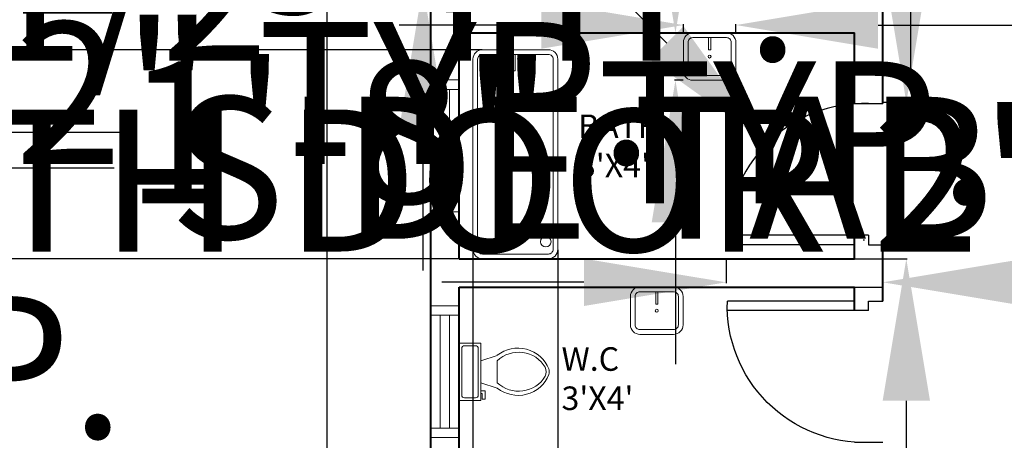
# Model space of a CAD drawing. Units: inches. Extents: x 7323 to 9737, y 2037 to 3322.
# Tile 8 of 19: x 8921 to 9130, y 2337 to 2426. Entities that reach past the tile are written whole.
import ezdxf

# ---------------------------------------------------------------- set-up
doc = ezdxf.new("R2010")
doc.units = ezdxf.units.IN
doc.header["$MEASUREMENT"] = 0
for name, color, linetype, lineweight in [('A-ANNO-DIMS', 2, 'Continuous', 18), ('A-AREA-IDEN', 7, 'Continuous', 18), ('A-DOOR', 4, 'Continuous', 25), ('A-FLOR-FIXT', 9, 'Continuous', 18), ('A-GLAZ', 4, 'Continuous', 18), ('A-WALL', 7, 'Continuous', 40)]:
    doc.layers.add(name, color=color, linetype=linetype, lineweight=lineweight)
doc.styles.get("Standard").update_dxf_attribs({"font": 'arial.ttf'})
doc.dimstyles.get("Standard").update_dxf_attribs({"dimtxt": 30.18, "dimasz": 30.18, "dimexe": 0.18, "dimexo": 0.0625, "dimgap": 0.09, "dimtad": 0, "dimtih": 1, "dimtoh": 1, "dimdec": 0, "dimzin": 0, "dimdsep": 46, "dimlunit": 3, "dimtxsty": 'Standard', "dimcen": 0.09, "dimadec": 0, "dimazin": 0, "dimtfac": 1, "dimtdec": 0, "dimtofl": 0, "dimtmove": 0, "dimatfit": 3, "dimfxl": 1, "dimtolj": 1, "dimtzin": 0, "dimarcsym": 0})

# ---------------------------------------------------------------- blocks, each defined once
blk = doc.blocks.new('*U2')
for p, q in [((9.5, -6), (9.5, -2)), ((-10, -8.5), (-8, -8.5)), ((-10, -9.5), (-10, -8.5)), ((-7, -9.5), (-10, -9.5)), ((-8, -8.5), (-8, -8)), ((-7, -8), (-7, -9.5)), ((-4, -8), (-6, -14)), ((4, -8), (6, -14)), ((4, -14), (-4, -14))]:
    blk.add_line(p, q)
blk.add_lwpolyline([(10.5, -8), (10.5, 0), (-10.5, 0), (-10.5, -8)], close=True)
for points in [[(-9.5, -2), (-9.5, -6)], [(8.5, -1), (-8.5, -1)], [(-8.5, -7), (8.5, -7)]]:
    blk.add_lwpolyline(points)
for centre, radius, start, end in [((-8.62, -1.88), 0.884, 81.8699, 188.1301), ((8.62, -1.88), 0.884, 351.8699, 98.1301), ((-8.62, -6.12), 0.884, 171.8699, 278.1301), ((8.62, -6.12), 0.884, 261.8699, 8.1301), ((3.52, -21.58), 12.17, 141.4691, 247.9714), ((4.2, -21.82), 11.33, 136.3677, 238.9468), ((-3.52, -21.58), 12.17, 292.0284, 38.5307), ((-4.2, -21.82), 11.33, 301.053, 43.6321), ((0, -27.88), 4, 245.7318, 294.2682), ((0, -29), 4, 254.8605, 285.1395)]:
    blk.add_arc(centre, radius, start, end)
blk = doc.blocks.new('*D11')
at = {"layer": 'A-ANNO-DIMS', "color": 0, "lineweight": -2, "transparency": 16777216}
for p, q in [((9007.88, 2687.3), (8985.8, 2687.3)), ((8985.98, 2657.12), (8985.98, 2458.79)), ((8985.98, 2229.48), (8985.98, 2427.8)), ((9007.88, 2199.3), (8985.8, 2199.3))]:
    blk.add_line(p, q, dxfattribs=at)
at = {"layer": 'A-ANNO-DIMS', "color": 0, "transparency": 16777216}
for points in [[(8980.95, 2657.12), (8991.01, 2657.12), (8985.98, 2687.3)], [(8980.95, 2229.48), (8991.01, 2229.48), (8985.98, 2199.3)]]:
    blk.add_solid(points, dxfattribs=at)
at = {"layer": 'Defpoints', "color": 0, "transparency": 16777216}
for p in [(9007.95, 2687.3), (8985.98, 2199.3), (9007.95, 2199.3)]:
    blk.add_point(p, dxfattribs=at)
at = {"layer": 'A-ANNO-DIMS', "color": 0, "transparency": 16777216, "insert": (8985.98, 2443.3), "char_height": 30.18, "attachment_point": 5}
blk.add_mtext('\\A1;40\'-8"', dxfattribs=at)
blk = doc.blocks.new('WIN-24')
for p, q in [((6, 28), (0, 28)), ((6, 26), (0, 26)), ((2, 26), (2, 2)), ((4, 26), (4, 2)), ((6, 2), (0, 2)), ((6, 0), (0, 0))]:
    blk.add_line(p, q)
blk = doc.blocks.new('DOOR-30')
for p, q in [((27.01, 33), (33.01, 33)), ((30.01, 5), (0.01, 5)), ((30.01, 5), (30.01, 3)), ((27.01, 3), (0.01, 3)), ((30.01, 3), (33.01, 3)), ((27.01, 0), (33.01, 0))]:
    blk.add_line(p, q)
blk.add_arc((29.01, 4), 29.02, 88.0251, 181.9749)
blk = doc.blocks.new('BASIN-WALL-MOUNT')
for points in [[(0, 8.06, -0.414214), (2, 10.06), (9.16, 10.06, -0.414214), (11.16, 8.06), (11.16, 2, -0.414214), (9.16, 0), (2, 0, -0.414214), (0, 2)], [(1, 8.06, -0.414214), (2, 9.06), (9.16, 9.06, -0.414214), (10.16, 8.06), (10.16, 2, -0.414214), (9.16, 1), (2, 1, -0.414214), (1, 2)]]:
    blk.add_lwpolyline(points, format="xyb", close=True)
blk.add_lwpolyline([(5.83, 9.06), (5.83, 9.06), (5.37, 9.06), (5.37, 9.06), (5.37, 6.45), (5.37, 6.45), (5.83, 6.45), (5.83, 6.45)], close=True)
blk.add_circle((5.58, 5.03), 0.311)
blk = doc.blocks.new('*D41')
at = {"layer": 'A-ANNO-DIMS', "color": 0, "lineweight": -2, "transparency": 16777216}
for p, q in [((8661.59, 2428.04), (8661.59, 2458.22)), ((8661.59, 2458.22), (8691.77, 2458.22)), ((8657.46, 2397.86), (8661.77, 2397.86)), ((8657.46, 2369.86), (8661.77, 2369.86)), ((8661.59, 2339.68), (8661.59, 2309.5))]:
    blk.add_line(p, q, dxfattribs=at)
at = {"layer": 'A-ANNO-DIMS', "color": 0, "transparency": 16777216}
for points in [[(8656.56, 2428.04), (8666.62, 2428.04), (8661.59, 2397.86)], [(8656.56, 2339.68), (8666.62, 2339.68), (8661.59, 2369.86)]]:
    blk.add_solid(points, dxfattribs=at)
at = {"layer": 'Defpoints', "color": 0, "transparency": 16777216}
for p in [(8657.39, 2397.86), (8661.59, 2397.86), (8657.39, 2369.86)]:
    blk.add_point(p, dxfattribs=at)
at = {"layer": 'A-ANNO-DIMS', "color": 0, "transparency": 16777216, "insert": (8945.06, 2458.22), "char_height": 30.18, "attachment_point": 5}
blk.add_mtext('\\A1;VENT WINDOW 2\'-4" TYP.', dxfattribs=at)
blk = doc.blocks.new('*D43')
at = {"layer": 'A-ANNO-DIMS', "color": 0, "lineweight": -2, "transparency": 16777216}
for p, q in [((9108.94, 2438.75), (9108.94, 2468.93)), ((9104.01, 2408.57), (9109.12, 2408.57)), ((9104.01, 2375.3), (9109.12, 2375.3)), ((9108.94, 2345.12), (9108.94, 2314.94))]:
    blk.add_line(p, q, dxfattribs=at)
at = {"layer": 'A-ANNO-DIMS', "color": 0, "transparency": 16777216}
for points in [[(9103.91, 2438.75), (9113.97, 2438.75), (9108.94, 2408.57)], [(9103.91, 2345.12), (9113.97, 2345.12), (9108.94, 2375.3)]]:
    blk.add_solid(points, dxfattribs=at)
at = {"layer": 'Defpoints', "color": 0, "transparency": 16777216}
for p in [(9103.95, 2408.57), (9108.94, 2408.57), (9103.95, 2375.3)]:
    blk.add_point(p, dxfattribs=at)
at = {"layer": 'A-ANNO-DIMS', "color": 0, "transparency": 16777216, "insert": (9108.94, 2391.93), "char_height": 30.18, "attachment_point": 5}
blk.add_mtext('\\A1;BATH DOOR 2\'-9 1/2" TYP.', dxfattribs=at)
blk = doc.blocks.new('*D44')
at = {"layer": 'A-ANNO-DIMS', "color": 0, "lineweight": -2, "transparency": 16777216}
for p, q in [((9070.67, 2375.23), (9070.67, 2370.12)), ((9103.95, 2375.23), (9103.95, 2370.12)), ((9040.49, 2370.3), (9010.31, 2370.3)), ((9134.13, 2370.3), (9164.31, 2370.3))]:
    blk.add_line(p, q, dxfattribs=at)
at = {"layer": 'A-ANNO-DIMS', "color": 0, "transparency": 16777216}
for points in [[(9040.49, 2375.33), (9040.49, 2365.27), (9070.67, 2370.3)], [(9134.13, 2375.33), (9134.13, 2365.27), (9103.95, 2370.3)]]:
    blk.add_solid(points, dxfattribs=at)
at = {"layer": 'Defpoints', "color": 0, "transparency": 16777216}
for p in [(9070.67, 2375.3), (9103.95, 2375.3), (9103.95, 2370.3)]:
    blk.add_point(p, dxfattribs=at)
at = {"layer": 'A-ANNO-DIMS', "color": 0, "transparency": 16777216, "insert": (9291.8, 2370.3), "char_height": 30.18, "attachment_point": 5}
blk.add_mtext('\\A1;2\'-9 1/2" TYP.', dxfattribs=at)
blk = doc.blocks.new('*D47')
at = {"layer": 'A-ANNO-DIMS', "color": 0, "lineweight": -2, "transparency": 16777216}
for p, q in [((8809.55, 2464.49), (8779.37, 2464.49)), ((8839.73, 2461.79), (8839.73, 2464.67)), ((8858.14, 2461.79), (8858.14, 2464.67)), ((8888.32, 2464.49), (8918.5, 2464.49))]:
    blk.add_line(p, q, dxfattribs=at)
at = {"layer": 'A-ANNO-DIMS', "color": 0, "transparency": 16777216}
for points in [[(8809.55, 2469.52), (8809.55, 2459.46), (8839.73, 2464.49)], [(8888.32, 2469.52), (8888.32, 2459.46), (8858.14, 2464.49)]]:
    blk.add_solid(points, dxfattribs=at)
at = {"layer": 'Defpoints', "color": 0, "transparency": 16777216}
for p in [(8858.14, 2464.49), (8839.73, 2461.73), (8858.14, 2461.73)]:
    blk.add_point(p, dxfattribs=at)
at = {"layer": 'A-ANNO-DIMS', "color": 0, "transparency": 16777216, "insert": (9164.9, 2464.49), "char_height": 30.18, "attachment_point": 5}
blk.add_mtext('\\A1;ARMCHAIR 1\'-6 1/2" TYP.', dxfattribs=at)
blk = doc.blocks.new('*D48')
at = {"layer": 'A-ANNO-DIMS', "color": 0, "lineweight": -2, "transparency": 16777216}
for p, q in [((8836.96, 2491.91), (8836.96, 2522.09)), ((8836.96, 2522.09), (8867.14, 2522.09)), ((8839.66, 2461.73), (8836.78, 2461.73)), ((8839.66, 2451.75), (8836.78, 2451.75)), ((8836.96, 2421.57), (8836.96, 2391.39))]:
    blk.add_line(p, q, dxfattribs=at)
at = {"layer": 'A-ANNO-DIMS', "color": 0, "transparency": 16777216}
for points in [[(8831.93, 2491.91), (8841.99, 2491.91), (8836.96, 2461.73)], [(8831.93, 2421.57), (8841.99, 2421.57), (8836.96, 2451.75)]]:
    blk.add_solid(points, dxfattribs=at)
at = {"layer": 'Defpoints', "color": 0, "transparency": 16777216}
for p in [(8836.96, 2461.73), (8839.73, 2461.73), (8839.73, 2451.75)]:
    blk.add_point(p, dxfattribs=at)
at = {"layer": 'A-ANNO-DIMS', "color": 0, "transparency": 16777216, "insert": (8970.94, 2522.09), "char_height": 30.18, "attachment_point": 5}
blk.add_mtext('\\A1;0\'-10" TYP.', dxfattribs=at)
blk = doc.blocks.new('*D53')
at = {"layer": 'A-ANNO-DIMS', "color": 0, "lineweight": -2, "transparency": 16777216}
for p, q in [((8857.03, 2503.93), (8857.03, 2511.24)), ((8905.03, 2503.93), (8905.03, 2511.24)), ((8826.85, 2511.06), (8796.67, 2511.06)), ((8935.21, 2511.06), (8965.39, 2511.06))]:
    blk.add_line(p, q, dxfattribs=at)
at = {"layer": 'A-ANNO-DIMS', "color": 0, "transparency": 16777216}
for points in [[(8826.85, 2516.09), (8826.85, 2506.03), (8857.03, 2511.06)], [(8935.21, 2516.09), (8935.21, 2506.03), (8905.03, 2511.06)]]:
    blk.add_solid(points, dxfattribs=at)
at = {"layer": 'Defpoints', "color": 0, "transparency": 16777216}
for p in [(8905.03, 2511.06), (8857.03, 2503.86), (8905.03, 2503.86)]:
    blk.add_point(p, dxfattribs=at)
at = {"layer": 'A-ANNO-DIMS', "color": 0, "transparency": 16777216, "insert": (9261.3, 2511.06), "char_height": 30.18, "attachment_point": 5}
blk.add_mtext('\\A1;INTERIOR WINDOW 4\'-0" TYP.', dxfattribs=at)
blk = doc.blocks.new('*D55')
at = {"layer": 'A-ANNO-DIMS', "color": 0, "lineweight": -2, "transparency": 16777216}
for p, q in [((9265.38, 2351.3), (9282, 2351.3)), ((9281.82, 2321.12), (9281.82, 2311.99)), ((9281.82, 2271.48), (9281.82, 2280.6)), ((9265.38, 2241.3), (9282, 2241.3))]:
    blk.add_line(p, q, dxfattribs=at)
at = {"layer": 'A-ANNO-DIMS', "color": 0, "transparency": 16777216}
for points in [[(9276.79, 2321.12), (9286.85, 2321.12), (9281.82, 2351.3)], [(9276.79, 2271.48), (9286.85, 2271.48), (9281.82, 2241.3)]]:
    blk.add_solid(points, dxfattribs=at)
at = {"layer": 'Defpoints', "color": 0, "transparency": 16777216}
for p in [(9265.32, 2351.3), (9281.82, 2351.3), (9265.32, 2241.3)]:
    blk.add_point(p, dxfattribs=at)
at = {"layer": 'A-ANNO-DIMS', "color": 0, "transparency": 16777216, "insert": (9281.82, 2296.3), "char_height": 30.18, "attachment_point": 5}
blk.add_mtext('\\A1;STAIR FLIGHT 9\'-2" TYP.', dxfattribs=at)
blk = doc.blocks.new('*D59')
at = {"layer": 'A-ANNO-DIMS', "color": 0, "lineweight": -2, "transparency": 16777216}
for p, q in [((9064.67, 2473.96), (9064.67, 2467.95)), ((9103.95, 2473.96), (9103.95, 2467.95)), ((9034.49, 2468.13), (9004.31, 2468.13)), ((9134.13, 2468.13), (9164.31, 2468.13))]:
    blk.add_line(p, q, dxfattribs=at)
at = {"layer": 'A-ANNO-DIMS', "color": 0, "transparency": 16777216}
for points in [[(9034.49, 2473.16), (9034.49, 2463.1), (9064.67, 2468.13)], [(9134.13, 2473.16), (9134.13, 2463.1), (9103.95, 2468.13)]]:
    blk.add_solid(points, dxfattribs=at)
at = {"layer": 'Defpoints', "color": 0, "transparency": 16777216}
for p in [(9064.67, 2474.02), (9103.95, 2474.02), (9103.95, 2468.13)]:
    blk.add_point(p, dxfattribs=at)
at = {"layer": 'A-ANNO-DIMS', "color": 0, "transparency": 16777216, "insert": (9458.35, 2468.13), "char_height": 30.18, "attachment_point": 5}
blk.add_mtext('\\A1;KITCHEN DOOR 3\'-3 1/2" TYP.', dxfattribs=at)
blk = doc.blocks.new('*D60')
at = {"layer": 'A-ANNO-DIMS', "color": 0, "lineweight": -2, "transparency": 16777216}
for p, q in [((9109.84, 2540.48), (9109.84, 2570.66)), ((9104.01, 2510.3), (9110.02, 2510.3)), ((9104.01, 2474.02), (9110.02, 2474.02)), ((9109.84, 2443.84), (9109.84, 2413.66))]:
    blk.add_line(p, q, dxfattribs=at)
at = {"layer": 'A-ANNO-DIMS', "color": 0, "transparency": 16777216}
for points in [[(9104.81, 2540.48), (9114.87, 2540.48), (9109.84, 2510.3)], [(9104.81, 2443.84), (9114.87, 2443.84), (9109.84, 2474.02)]]:
    blk.add_solid(points, dxfattribs=at)
at = {"layer": 'Defpoints', "color": 0, "transparency": 16777216}
for p in [(9103.95, 2510.3), (9109.84, 2510.3), (9103.95, 2474.02)]:
    blk.add_point(p, dxfattribs=at)
at = {"layer": 'A-ANNO-DIMS', "color": 0, "transparency": 16777216, "insert": (9109.84, 2492.16), "char_height": 30.18, "attachment_point": 5}
blk.add_mtext('\\A1;3\'-0 1/2" TYP.', dxfattribs=at)
blk = doc.blocks.new('*D63')
at = {"layer": 'A-ANNO-DIMS', "color": 0, "lineweight": -2, "transparency": 16777216}
for p, q in [((8744.72, 2466.22), (8744.72, 2496.4)), ((8744.72, 2496.4), (8774.9, 2496.4)), ((8741.46, 2436.04), (8744.9, 2436.04)), ((8741.46, 2413.86), (8744.9, 2413.86)), ((8744.72, 2383.68), (8744.72, 2353.5))]:
    blk.add_line(p, q, dxfattribs=at)
at = {"layer": 'A-ANNO-DIMS', "color": 0, "transparency": 16777216}
for points in [[(8739.69, 2466.22), (8749.75, 2466.22), (8744.72, 2436.04)], [(8739.69, 2383.68), (8749.75, 2383.68), (8744.72, 2413.86)]]:
    blk.add_solid(points, dxfattribs=at)
at = {"layer": 'Defpoints', "color": 0, "transparency": 16777216}
for p in [(8741.39, 2436.04), (8744.72, 2436.04), (8741.39, 2413.86)]:
    blk.add_point(p, dxfattribs=at)
at = {"layer": 'A-ANNO-DIMS', "color": 0, "transparency": 16777216, "insert": (9003.76, 2496.4), "char_height": 30.18, "attachment_point": 5}
blk.add_mtext('\\A1;APPLIANCE 1\'-10" TYP.', dxfattribs=at)
blk = doc.blocks.new('*D64')
at = {"layer": 'A-ANNO-DIMS', "color": 0, "lineweight": -2, "transparency": 16777216}
for p, q in [((8719.69, 2413.8), (8719.69, 2410.36)), ((8741.39, 2413.8), (8741.39, 2410.36)), ((8689.51, 2410.54), (8659.33, 2410.54)), ((8771.57, 2410.54), (8801.75, 2410.54))]:
    blk.add_line(p, q, dxfattribs=at)
at = {"layer": 'A-ANNO-DIMS', "color": 0, "transparency": 16777216}
for points in [[(8689.51, 2415.57), (8689.51, 2405.51), (8719.69, 2410.54)], [(8771.57, 2415.57), (8771.57, 2405.51), (8741.39, 2410.54)]]:
    blk.add_solid(points, dxfattribs=at)
at = {"layer": 'Defpoints', "color": 0, "transparency": 16777216}
for p in [(8719.69, 2413.86), (8741.39, 2413.86), (8741.39, 2410.54)]:
    blk.add_point(p, dxfattribs=at)
at = {"layer": 'A-ANNO-DIMS', "color": 0, "transparency": 16777216, "insert": (8927.57, 2410.54), "char_height": 30.18, "attachment_point": 5}
blk.add_mtext('\\A1;1\'-9 1/2" TYP.', dxfattribs=at)
blk = doc.blocks.new('*D67')
at = {"layer": 'A-ANNO-DIMS', "color": 0, "lineweight": -2, "transparency": 16777216}
for p, q in [((9145.07, 2308.82), (9145.07, 2339)), ((9150.37, 2278.64), (9144.89, 2278.64)), ((9150.37, 2242.89), (9144.89, 2242.89)), ((9145.07, 2212.71), (9145.07, 2182.53))]:
    blk.add_line(p, q, dxfattribs=at)
at = {"layer": 'A-ANNO-DIMS', "color": 0, "transparency": 16777216}
for points in [[(9140.04, 2308.82), (9150.1, 2308.82), (9145.07, 2278.64)], [(9140.04, 2212.71), (9150.1, 2212.71), (9145.07, 2242.89)]]:
    blk.add_solid(points, dxfattribs=at)
at = {"layer": 'Defpoints', "color": 0, "transparency": 16777216}
for p in [(9145.07, 2278.64), (9150.44, 2278.64), (9150.44, 2242.89)]:
    blk.add_point(p, dxfattribs=at)
at = {"layer": 'A-ANNO-DIMS', "color": 0, "transparency": 16777216, "insert": (9145.07, 2260.76), "char_height": 30.18, "attachment_point": 5}
blk.add_mtext('\\A1;TV UNIT 2\'-11 1/2" TYP.', dxfattribs=at)
blk = doc.blocks.new('*D68')
at = {"layer": 'A-ANNO-DIMS', "color": 0, "lineweight": -2, "transparency": 16777216}
for p, q in [((9120.26, 2284), (9090.08, 2284)), ((9150.44, 2278.7), (9150.44, 2284.18)), ((9163.95, 2278.7), (9163.95, 2284.18)), ((9194.13, 2284), (9224.31, 2284))]:
    blk.add_line(p, q, dxfattribs=at)
at = {"layer": 'A-ANNO-DIMS', "color": 0, "transparency": 16777216}
for points in [[(9120.26, 2289.03), (9120.26, 2278.97), (9150.44, 2284)], [(9194.13, 2289.03), (9194.13, 2278.97), (9163.95, 2284)]]:
    blk.add_solid(points, dxfattribs=at)
at = {"layer": 'Defpoints', "color": 0, "transparency": 16777216}
for p in [(9163.95, 2284), (9150.44, 2278.64), (9163.95, 2278.64)]:
    blk.add_point(p, dxfattribs=at)
at = {"layer": 'A-ANNO-DIMS', "color": 0, "transparency": 16777216, "insert": (9350.12, 2284), "char_height": 30.18, "attachment_point": 5}
blk.add_mtext('\\A1;1\'-1 1/2" TYP.', dxfattribs=at)
blk = doc.blocks.new('*D69')
at = {"layer": 'A-ANNO-DIMS', "color": 0, "lineweight": -2, "transparency": 16777216}
for p, q in [((8836.58, 2472.89), (8836.58, 2503.07)), ((8836.58, 2503.07), (8866.76, 2503.07)), ((8839.88, 2442.71), (8836.4, 2442.71)), ((8839.88, 2420.33), (8836.4, 2420.33)), ((8836.58, 2390.15), (8836.58, 2359.97))]:
    blk.add_line(p, q, dxfattribs=at)
at = {"layer": 'A-ANNO-DIMS', "color": 0, "transparency": 16777216}
for points in [[(8831.55, 2472.89), (8841.61, 2472.89), (8836.58, 2442.71)], [(8831.55, 2390.15), (8841.61, 2390.15), (8836.58, 2420.33)]]:
    blk.add_solid(points, dxfattribs=at)
at = {"layer": 'Defpoints', "color": 0, "transparency": 16777216}
for p in [(8836.58, 2442.71), (8839.94, 2442.71), (8839.94, 2420.33)]:
    blk.add_point(p, dxfattribs=at)
at = {"layer": 'A-ANNO-DIMS', "color": 0, "transparency": 16777216, "insert": (9169.54, 2503.07), "char_height": 30.18, "attachment_point": 5}
blk.add_mtext('\\A1;COFFEE TABLE 1\'-10 1/2" TYP.', dxfattribs=at)
blk = doc.blocks.new('*D70')
at = {"layer": 'A-ANNO-DIMS', "color": 0, "lineweight": -2, "transparency": 16777216}
for p, q in [((8809.76, 2446.06), (8779.58, 2446.06)), ((8839.94, 2442.77), (8839.94, 2446.24)), ((8855.74, 2442.77), (8855.74, 2446.24)), ((8885.92, 2446.06), (8916.1, 2446.06))]:
    blk.add_line(p, q, dxfattribs=at)
at = {"layer": 'A-ANNO-DIMS', "color": 0, "transparency": 16777216}
for points in [[(8809.76, 2451.09), (8809.76, 2441.03), (8839.94, 2446.06)], [(8885.92, 2451.09), (8885.92, 2441.03), (8855.74, 2446.06)]]:
    blk.add_solid(points, dxfattribs=at)
at = {"layer": 'Defpoints', "color": 0, "transparency": 16777216}
for p in [(8855.74, 2446.06), (8839.94, 2442.71), (8855.74, 2442.71)]:
    blk.add_point(p, dxfattribs=at)
at = {"layer": 'A-ANNO-DIMS', "color": 0, "transparency": 16777216, "insert": (9006.75, 2446.06), "char_height": 30.18, "attachment_point": 5}
blk.add_mtext('\\A1;1\'-4" TYP.', dxfattribs=at)
blk = doc.blocks.new('*D71')
at = {"layer": 'A-ANNO-DIMS', "color": 0, "lineweight": -2, "transparency": 16777216}
for p, q in [((8891.18, 2486.02), (8891.18, 2516.2)), ((8884.24, 2455.84), (8891.36, 2455.84)), ((8884.24, 2409.18), (8891.36, 2409.18)), ((8891.18, 2379), (8891.18, 2348.82))]:
    blk.add_line(p, q, dxfattribs=at)
at = {"layer": 'A-ANNO-DIMS', "color": 0, "transparency": 16777216}
for points in [[(8886.15, 2486.02), (8896.21, 2486.02), (8891.18, 2455.84)], [(8886.15, 2379), (8896.21, 2379), (8891.18, 2409.18)]]:
    blk.add_solid(points, dxfattribs=at)
at = {"layer": 'Defpoints', "color": 0, "transparency": 16777216}
for p in [(8884.18, 2455.84), (8891.18, 2455.84), (8884.18, 2409.18)]:
    blk.add_point(p, dxfattribs=at)
at = {"layer": 'A-ANNO-DIMS', "color": 0, "transparency": 16777216, "insert": (8891.18, 2432.51), "char_height": 30.18, "attachment_point": 5}
blk.add_mtext('\\A1;SOFA 3\'-10 1/2" TYP.', dxfattribs=at)
blk = doc.blocks.new('*D72')
at = {"layer": 'A-ANNO-DIMS', "color": 0, "lineweight": -2, "transparency": 16777216}
for p, q in [((8864.06, 2409.12), (8864.06, 2402)), ((8884.18, 2409.12), (8884.18, 2402)), ((8833.88, 2402.18), (8803.7, 2402.18)), ((8914.36, 2402.18), (8944.54, 2402.18))]:
    blk.add_line(p, q, dxfattribs=at)
at = {"layer": 'A-ANNO-DIMS', "color": 0, "transparency": 16777216}
for points in [[(8833.88, 2407.21), (8833.88, 2397.15), (8864.06, 2402.18)], [(8914.36, 2407.21), (8914.36, 2397.15), (8884.18, 2402.18)]]:
    blk.add_solid(points, dxfattribs=at)
at = {"layer": 'Defpoints', "color": 0, "transparency": 16777216}
for p in [(8864.06, 2409.18), (8884.18, 2409.18), (8884.18, 2402.18)]:
    blk.add_point(p, dxfattribs=at)
at = {"layer": 'A-ANNO-DIMS', "color": 0, "transparency": 16777216, "insert": (9035.19, 2402.18), "char_height": 30.18, "attachment_point": 5}
blk.add_mtext('\\A1;1\'-8" TYP.', dxfattribs=at)
blk = doc.blocks.new('*D73')
at = {"layer": 'A-ANNO-DIMS', "color": 0, "lineweight": -2, "transparency": 16777216}
for p, q in [((9031.41, 2424.97), (9001.23, 2424.97)), ((9061.59, 2423.36), (9061.59, 2425.15)), ((9072.75, 2423.36), (9072.75, 2425.15)), ((9102.93, 2424.97), (9133.11, 2424.97))]:
    blk.add_line(p, q, dxfattribs=at)
at = {"layer": 'A-ANNO-DIMS', "color": 0, "transparency": 16777216}
for points in [[(9031.41, 2430), (9031.41, 2419.94), (9061.59, 2424.97)], [(9102.93, 2430), (9102.93, 2419.94), (9072.75, 2424.97)]]:
    blk.add_solid(points, dxfattribs=at)
at = {"layer": 'Defpoints', "color": 0, "transparency": 16777216}
for p in [(9072.75, 2424.97), (9061.59, 2423.3), (9072.75, 2423.3)]:
    blk.add_point(p, dxfattribs=at)
at = {"layer": 'A-ANNO-DIMS', "color": 0, "transparency": 16777216, "insert": (9305.36, 2424.97), "char_height": 30.18, "attachment_point": 5}
blk.add_mtext('\\A1;BASIN 0\'-11" TYP.', dxfattribs=at)
blk = doc.blocks.new('*D74')
at = {"layer": 'A-ANNO-DIMS', "color": 0, "lineweight": -2, "transparency": 16777216}
for p, q in [((9059.91, 2453.48), (9059.91, 2483.66)), ((9059.91, 2483.66), (9090.09, 2483.66)), ((9061.53, 2423.3), (9059.73, 2423.3)), ((9061.53, 2413.24), (9059.73, 2413.24)), ((9059.91, 2383.06), (9059.91, 2352.88))]:
    blk.add_line(p, q, dxfattribs=at)
at = {"layer": 'A-ANNO-DIMS', "color": 0, "transparency": 16777216}
for points in [[(9054.88, 2453.48), (9064.94, 2453.48), (9059.91, 2423.3)], [(9054.88, 2383.06), (9064.94, 2383.06), (9059.91, 2413.24)]]:
    blk.add_solid(points, dxfattribs=at)
at = {"layer": 'Defpoints', "color": 0, "transparency": 16777216}
for p in [(9059.91, 2423.3), (9061.59, 2423.3), (9061.59, 2413.24)]:
    blk.add_point(p, dxfattribs=at)
at = {"layer": 'A-ANNO-DIMS', "color": 0, "transparency": 16777216, "insert": (9193.89, 2483.66), "char_height": 30.18, "attachment_point": 5}
blk.add_mtext('\\A1;0\'-10" TYP.', dxfattribs=at)
blk = doc.blocks.new('*D75')
at = {"layer": 'A-ANNO-DIMS', "color": 0, "lineweight": -2, "transparency": 16777216}
for p, q in [((8629.63, 2293.84), (8599.45, 2293.84)), ((8659.81, 2292), (8659.81, 2294.02)), ((8672.52, 2292), (8672.52, 2294.02)), ((8702.7, 2293.84), (8732.88, 2293.84))]:
    blk.add_line(p, q, dxfattribs=at)
at = {"layer": 'A-ANNO-DIMS', "color": 0, "transparency": 16777216}
for points in [[(8629.63, 2298.87), (8629.63, 2288.81), (8659.81, 2293.84)], [(8702.7, 2298.87), (8702.7, 2288.81), (8672.52, 2293.84)]]:
    blk.add_solid(points, dxfattribs=at)
at = {"layer": 'Defpoints', "color": 0, "transparency": 16777216}
for p in [(8672.52, 2293.84), (8659.81, 2291.93), (8672.52, 2291.93)]:
    blk.add_point(p, dxfattribs=at)
at = {"layer": 'A-ANNO-DIMS', "color": 0, "transparency": 16777216, "insert": (9002.27, 2293.84), "char_height": 30.18, "attachment_point": 5}
blk.add_mtext('\\A1;NIGHTSTAND 1\'-0 1/2" TYP.', dxfattribs=at)
blk = doc.blocks.new('*D76')
at = {"layer": 'A-ANNO-DIMS', "color": 0, "lineweight": -2, "transparency": 16777216}
for p, q in [((8657.91, 2322.11), (8657.91, 2352.29)), ((8657.91, 2352.29), (8688.09, 2352.29)), ((8659.75, 2291.93), (8657.73, 2291.93)), ((8659.75, 2282.32), (8657.73, 2282.32)), ((8657.91, 2252.14), (8657.91, 2221.96))]:
    blk.add_line(p, q, dxfattribs=at)
at = {"layer": 'A-ANNO-DIMS', "color": 0, "transparency": 16777216}
for points in [[(8652.88, 2322.11), (8662.94, 2322.11), (8657.91, 2291.93)], [(8652.88, 2252.14), (8662.94, 2252.14), (8657.91, 2282.32)]]:
    blk.add_solid(points, dxfattribs=at)
at = {"layer": 'Defpoints', "color": 0, "transparency": 16777216}
for p in [(8657.91, 2291.93), (8659.81, 2291.93), (8659.81, 2282.32)]:
    blk.add_point(p, dxfattribs=at)
at = {"layer": 'A-ANNO-DIMS', "color": 0, "transparency": 16777216, "insert": (8815.32, 2352.29), "char_height": 30.18, "attachment_point": 5}
blk.add_mtext('\\A1;0\'-9 1/2" TYP.', dxfattribs=at)
blk = doc.blocks.new('*D78')
at = {"layer": 'A-ANNO-DIMS', "color": 0, "lineweight": -2, "transparency": 16777216}
for p, q in [((9030.98, 2259.48), (9030.98, 2289.66)), ((9030.98, 2289.66), (9061.16, 2289.66)), ((9029.14, 2229.3), (9031.16, 2229.3)), ((9029.14, 2219.69), (9031.16, 2219.69)), ((9030.98, 2189.51), (9030.98, 2159.33))]:
    blk.add_line(p, q, dxfattribs=at)
at = {"layer": 'A-ANNO-DIMS', "color": 0, "transparency": 16777216}
for points in [[(9025.95, 2259.48), (9036.01, 2259.48), (9030.98, 2229.3)], [(9025.95, 2189.51), (9036.01, 2189.51), (9030.98, 2219.69)]]:
    blk.add_solid(points, dxfattribs=at)
at = {"layer": 'Defpoints', "color": 0, "transparency": 16777216}
for p in [(9029.07, 2229.3), (9030.98, 2229.3), (9029.07, 2219.69)]:
    blk.add_point(p, dxfattribs=at)
at = {"layer": 'A-ANNO-DIMS', "color": 0, "transparency": 16777216, "insert": (9188.39, 2289.66), "char_height": 30.18, "attachment_point": 5}
blk.add_mtext('\\A1;0\'-9 1/2" TYP.', dxfattribs=at)
blk = doc.blocks.new('*D79')
at = {"layer": 'A-ANNO-DIMS', "color": 0, "lineweight": -2, "transparency": 16777216}
for p, q in [((8840.92, 2394.64), (8810.74, 2394.64)), ((8871.1, 2395.97), (8871.1, 2394.46)), ((8880.36, 2395.97), (8880.36, 2394.46)), ((8910.54, 2394.64), (8940.72, 2394.64))]:
    blk.add_line(p, q, dxfattribs=at)
at = {"layer": 'A-ANNO-DIMS', "color": 0, "transparency": 16777216}
for points in [[(8840.92, 2399.67), (8840.92, 2389.61), (8871.1, 2394.64)], [(8910.54, 2399.67), (8910.54, 2389.61), (8880.36, 2394.64)]]:
    blk.add_solid(points, dxfattribs=at)
at = {"layer": 'Defpoints', "color": 0, "transparency": 16777216}
for p in [(8871.1, 2396.03), (8880.36, 2396.03), (8880.36, 2394.64)]:
    blk.add_point(p, dxfattribs=at)
at = {"layer": 'A-ANNO-DIMS', "color": 0, "transparency": 16777216, "insert": (9195.57, 2394.64), "char_height": 30.18, "attachment_point": 5}
blk.add_mtext('\\A1;SIDE TABLE 0\'-9 1/2" TYP.', dxfattribs=at)
blk = doc.blocks.new('*D80')
at = {"layer": 'A-ANNO-DIMS', "color": 0, "lineweight": -2, "transparency": 16777216}
for p, q in [((8881.74, 2435.12), (8881.74, 2465.3)), ((8881.74, 2465.3), (8911.92, 2465.3)), ((8880.42, 2404.94), (8881.92, 2404.94)), ((8880.42, 2396.03), (8881.92, 2396.03)), ((8881.74, 2365.85), (8881.74, 2335.67))]:
    blk.add_line(p, q, dxfattribs=at)
at = {"layer": 'A-ANNO-DIMS', "color": 0, "transparency": 16777216}
for points in [[(8876.71, 2435.12), (8886.77, 2435.12), (8881.74, 2404.94)], [(8876.71, 2365.85), (8886.77, 2365.85), (8881.74, 2396.03)]]:
    blk.add_solid(points, dxfattribs=at)
at = {"layer": 'Defpoints', "color": 0, "transparency": 16777216}
for p in [(8880.36, 2404.94), (8881.74, 2404.94), (8880.36, 2396.03)]:
    blk.add_point(p, dxfattribs=at)
at = {"layer": 'A-ANNO-DIMS', "color": 0, "transparency": 16777216, "insert": (9003.99, 2465.3), "char_height": 30.18, "attachment_point": 5}
blk.add_mtext('\\A1;0\'-9" TYP.', dxfattribs=at)
blk = doc.blocks.new('*D105')
at = {"layer": 'A-ANNO-DIMS', "color": 0, "lineweight": -2, "transparency": 16777216}
for p, q in [((9007.945402, 2365.232705), (9007.945402, 2148.482809)), ((9103.945402, 2333.232705), (9103.945402, 2148.482809)), ((8977.765402, 2148.662809), (8947.585402, 2148.662809)), ((9134.125402, 2148.662809), (9164.305402, 2148.662809))]:
    blk.add_line(p, q, dxfattribs=at)
at = {"layer": 'A-ANNO-DIMS', "color": 0, "transparency": 16777216}
for points in [[(8977.765402, 2153.692809), (8977.765402, 2143.632809), (9007.945402, 2148.662809)], [(9134.125402, 2153.692809), (9134.125402, 2143.632809), (9103.945402, 2148.662809)]]:
    blk.add_solid(points, dxfattribs=at)
at = {"layer": 'Defpoints', "color": 0, "transparency": 16777216}
for p in [(9007.945402, 2365.295205), (9103.945402, 2333.295205), (9103.945402, 2148.662809)]:
    blk.add_point(p, dxfattribs=at)
at = {"layer": 'A-ANNO-DIMS', "color": 0, "transparency": 16777216, "insert": (9055.945402, 2148.662809), "char_height": 30.18, "attachment_point": 5}
blk.add_mtext('\\A1;8\'-0"', dxfattribs=at)
blk = doc.blocks.new('*D106')
at = {"layer": 'A-ANNO-DIMS', "color": 0, "lineweight": -2, "transparency": 16777216}
for p, q in [((9008.12, 2519.31), (8587.16, 2519.31)), ((8587.34, 2489.13), (8587.34, 2439.14)), ((8587.34, 2357.76), (8587.34, 2407.75)), ((9008.23, 2327.58), (8587.16, 2327.58))]:
    blk.add_line(p, q, dxfattribs=at)
at = {"layer": 'A-ANNO-DIMS', "color": 0, "transparency": 16777216}
for points in [[(8582.31, 2489.13), (8592.37, 2489.13), (8587.34, 2519.31)], [(8582.31, 2357.76), (8592.37, 2357.76), (8587.34, 2327.58)]]:
    blk.add_solid(points, dxfattribs=at)
at = {"layer": 'Defpoints', "color": 0, "transparency": 16777216}
for p in [(8587.34, 2519.31), (9008.18, 2519.31), (9008.29, 2327.58)]:
    blk.add_point(p, dxfattribs=at)
at = {"layer": 'A-ANNO-DIMS', "color": 0, "transparency": 16777216, "insert": (8587.34, 2423.44), "char_height": 30.18, "attachment_point": 5}
blk.add_mtext('\\A1;15\'-11 1/2"', dxfattribs=at)
blk = doc.blocks.new('*D107')
at = {"layer": 'A-ANNO-DIMS', "color": 0, "lineweight": -2, "transparency": 16777216}
for p, q in [((8855.74, 2420.27), (8855.74, 2148.48)), ((8864.06, 2412.89), (8864.06, 2148.48)), ((8825.56, 2148.66), (8795.38, 2148.66)), ((8894.24, 2148.66), (8924.42, 2148.66))]:
    blk.add_line(p, q, dxfattribs=at)
at = {"layer": 'A-ANNO-DIMS', "color": 0, "transparency": 16777216}
for points in [[(8825.56, 2153.69), (8825.56, 2143.63), (8855.74, 2148.66)], [(8894.24, 2153.69), (8894.24, 2143.63), (8864.06, 2148.66)]]:
    blk.add_solid(points, dxfattribs=at)
at = {"layer": 'Defpoints', "color": 0, "transparency": 16777216}
for p in [(8855.74, 2420.33), (8864.06, 2412.95), (8864.06, 2148.66)]:
    blk.add_point(p, dxfattribs=at)
at = {"layer": 'A-ANNO-DIMS', "color": 0, "transparency": 16777216, "insert": (8999.78, 2148.66), "char_height": 30.18, "attachment_point": 5}
blk.add_mtext('\\A1;0\'-8 1/2"', dxfattribs=at)
blk = doc.blocks.new('*D109')
at = {"layer": 'A-ANNO-DIMS', "color": 0, "lineweight": -2, "transparency": 16777216}
for p, q in [((9016.91, 2377.23), (9016.91, 2148.48)), ((9034.93, 2377.23), (9034.93, 2148.48)), ((8986.73, 2148.66), (8956.55, 2148.66)), ((9065.11, 2148.66), (9095.29, 2148.66))]:
    blk.add_line(p, q, dxfattribs=at)
at = {"layer": 'A-ANNO-DIMS', "color": 0, "transparency": 16777216}
for points in [[(8986.73, 2153.69), (8986.73, 2143.63), (9016.91, 2148.66)], [(9065.11, 2153.69), (9065.11, 2143.63), (9034.93, 2148.66)]]:
    blk.add_solid(points, dxfattribs=at)
at = {"layer": 'Defpoints', "color": 0, "transparency": 16777216}
for p in [(9016.91, 2377.3), (9034.93, 2377.3), (9034.93, 2148.66)]:
    blk.add_point(p, dxfattribs=at)
at = {"layer": 'A-ANNO-DIMS', "color": 0, "transparency": 16777216, "insert": (9134.07, 2148.66), "char_height": 30.18, "attachment_point": 5}
blk.add_mtext('\\A1;1\'-6"', dxfattribs=at)
blk = doc.blocks.new('*D110')
at = {"layer": 'A-ANNO-DIMS', "color": 0, "lineweight": -2, "transparency": 16777216}
for p, q in [((8587.34, 2449.91), (8587.34, 2480.09)), ((9018.85, 2419.73), (8587.16, 2419.73)), ((9018.85, 2375.3), (8587.16, 2375.3)), ((8587.34, 2345.12), (8587.34, 2314.94))]:
    blk.add_line(p, q, dxfattribs=at)
at = {"layer": 'A-ANNO-DIMS', "color": 0, "transparency": 16777216}
for points in [[(8582.31, 2449.91), (8592.37, 2449.91), (8587.34, 2419.73)], [(8582.31, 2345.12), (8592.37, 2345.12), (8587.34, 2375.3)]]:
    blk.add_solid(points, dxfattribs=at)
at = {"layer": 'Defpoints', "color": 0, "transparency": 16777216}
for p in [(8587.34, 2419.73), (9018.91, 2419.73), (9018.91, 2375.3)]:
    blk.add_point(p, dxfattribs=at)
at = {"layer": 'A-ANNO-DIMS', "color": 0, "transparency": 16777216, "insert": (8587.34, 2397.51), "char_height": 30.18, "attachment_point": 5}
blk.add_mtext('\\A1;3\'-8 1/2"', dxfattribs=at)
blk = doc.blocks.new('*D112')
at = {"layer": 'A-ANNO-DIMS', "color": 0, "lineweight": -2, "transparency": 16777216}
for p, q in [((9006.28, 2476.47), (9006.28, 2506.65)), ((9006.28, 2506.65), (9036.46, 2506.65)), ((9041.42, 2446.29), (9006.1, 2446.29)), ((9041.42, 2433.19), (9006.1, 2433.19)), ((9006.28, 2403.01), (9006.28, 2372.83))]:
    blk.add_line(p, q, dxfattribs=at)
at = {"layer": 'A-ANNO-DIMS', "color": 0, "transparency": 16777216}
for points in [[(9001.25, 2476.47), (9011.31, 2476.47), (9006.28, 2446.29)], [(9001.25, 2403.01), (9011.31, 2403.01), (9006.28, 2433.19)]]:
    blk.add_solid(points, dxfattribs=at)
at = {"layer": 'Defpoints', "color": 0, "transparency": 16777216}
for p in [(9006.28, 2446.29), (9041.48, 2446.29), (9041.48, 2433.19)]:
    blk.add_point(p, dxfattribs=at)
at = {"layer": 'A-ANNO-DIMS', "color": 0, "transparency": 16777216, "insert": (9075.24, 2506.65), "char_height": 30.18, "attachment_point": 5}
blk.add_mtext('\\A1;1\'-1"', dxfattribs=at)
blk = doc.blocks.new('*D127')
at = {"layer": 'A-ANNO-DIMS', "color": 0, "lineweight": -2, "transparency": 16777216}
for p, q in [((9006.57, 2442.49), (9036.75, 2442.49)), ((9036.75, 2442.49), (9058.09, 2421.15)), ((9099.86, 2379.3), (9100.04, 2379.3)), ((9099.95, 2379.21), (9099.95, 2379.39))]:
    blk.add_line(p, q, dxfattribs=at)
at = {"layer": 'A-ANNO-DIMS', "color": 0, "transparency": 16777216}
blk.add_solid([(9061.64, 2424.71), (9054.53, 2417.6), (9079.43, 2399.81)], dxfattribs=at)
at = {"layer": 'Defpoints', "color": 0, "transparency": 16777216}
for p in [(9079.43, 2399.81), (9099.95, 2379.3)]:
    blk.add_point(p, dxfattribs=at)
at = {"layer": 'A-ANNO-DIMS', "color": 0, "transparency": 16777216, "insert": (8951.92, 2442.49), "char_height": 30.18, "attachment_point": 5}
blk.add_mtext('\\A1;R2\'-5"', dxfattribs=at)

msp = doc.modelspace()

# ---------------------------------------------------------------- linework, layer by layer
at = {"layer": 'A-FLOR-FIXT'}
for points in [[(9016.91, 2417.73, -0.414214), (9018.91, 2419.73), (9032.93, 2419.73, -0.414214), (9034.93, 2417.73), (9034.93, 2377.3, -0.414214), (9032.93, 2375.3), (9018.91, 2375.3, -0.414214), (9016.91, 2377.3)], [(9017.91, 2417.73, -0.414214), (9018.91, 2418.73), (9032.93, 2418.73, -0.414214), (9033.93, 2417.73), (9033.93, 2377.3, -0.414214), (9032.93, 2376.3), (9018.91, 2376.3, -0.414214), (9017.91, 2377.3)], [(9050.36, 2367.3, -0.414214), (9052.36, 2369.3), (9059.53, 2369.3, -0.414214), (9061.53, 2367.3), (9061.53, 2361.24, -0.414214), (9059.53, 2359.24), (9052.36, 2359.24, -0.414214), (9050.36, 2361.24)], [(9051.36, 2367.3, -0.414214), (9052.36, 2368.3), (9059.53, 2368.3, -0.414214), (9060.53, 2367.3), (9060.53, 2361.24, -0.414214), (9059.53, 2360.24), (9052.36, 2360.24, -0.414214), (9051.36, 2361.24)]]:
    msp.add_lwpolyline(points, format="xyb", close=True, dxfattribs=at)
for points in [[(9025.17, 2418.73), (9025.17, 2418.73), (9025.88, 2418.73), (9025.88, 2418.73), (9025.88, 2415.27), (9025.88, 2415.27), (9025.17, 2415.27), (9025.17, 2415.27)], [(9056.2, 2368.3), (9056.2, 2368.3), (9055.73, 2368.3), (9055.73, 2368.3), (9055.73, 2365.68), (9055.73, 2365.68), (9056.2, 2365.68), (9056.2, 2365.68)]]:
    msp.add_lwpolyline(points, close=True, dxfattribs=at)
for centre, radius in [((9024.43, 2417.82), 0.332), ((9026.7, 2417.79), 0.332), ((9032.38, 2378.93), 1.12), ((9055.95, 2364.27), 0.311)]:
    msp.add_circle(centre, radius, dxfattribs=at)
at = {"layer": 'A-WALL'}
for p, q in [((9007.95, 2199.3), (9007.95, 2687.3)), ((9103.95, 2408.3), (9103.95, 2474.3)), ((9103.95, 2423.3), (9103.95, 2474.3)), ((9013.95, 2375.3), (9013.95, 2423.3)), ((9013.95, 2423.3), (9097.95, 2423.3)), ((9097.95, 2408.24), (9097.95, 2423.3)), ((9097.95, 2375.3), (9097.95, 2380.3)), ((9103.95, 2366.3), (9103.95, 2378.3)), ((9013.95, 2375.3), (9097.95, 2375.3)), ((9013.95, 2333.3), (9013.95, 2369.3)), ((9013.95, 2369.3), (9097.95, 2369.3)), ((9097.95, 2364.3), (9097.95, 2369.3))]:
    msp.add_line(p, q, dxfattribs=at)

# ---------------------------------------------------------------- block references
at = {"layer": 'A-DOOR'}
msp.add_blockref('DOOR-30', (9070.93, 2375.3), dxfattribs=at)
at = {"layer": 'A-DOOR', "extrusion": (0, 0, -1), "zscale": -1, "rotation": 180}
msp.add_blockref('DOOR-30', (-9070.93, 2369.3), dxfattribs=at)
at = {"layer": 'A-FLOR-FIXT'}
msp.add_blockref('BASIN-WALL-MOUNT', (9061.59, 2413.24), dxfattribs=at)
at = {"layer": 'A-FLOR-FIXT', "xscale": 0.5808479307613652, "yscale": 0.5808479307613652, "zscale": 0.5808479307613652, "rotation": 90}
msp.add_blockref('*U2', (9013.95, 2351.3), dxfattribs=at)
at = {"layer": 'A-GLAZ', "rotation": 180}
for p in [(9013.95, 2413.3), (9013.95, 2365.3)]:
    msp.add_blockref('WIN-24', p, dxfattribs=at)

# ---------------------------------------------------------------- texts
at = {"layer": 'A-AREA-IDEN', "char_height": 5, "attachment_point": 1}
for s, insert in [("BATH\\P3'X4'", (9039.22, 2405.96)), ("W.C\\P3'X4'", (9035.72, 2356.5))]:
    msp.add_mtext_dynamic_manual_height_columns(s, width=44.1759, gutter_width=1, heights=[0], dxfattribs=dict(at, insert=insert))

# ---------------------------------------------------------------- dimensions: what is measured, and where the dimension line sits
at = {"layer": 'A-ANNO-DIMS'}
for base, p1, p2, override, picture, middle in [((8985.98, 2199.3), (9007.95, 2687.3), (9007.95, 2199.3), {"dimclrd": 0, "dimclre": 0, "dimclrt": 0}, '*D11', (8985.98, 2443.3)), ((9006.28, 2446.29), (9041.48, 2433.19), (9041.48, 2446.29), {"dimdec": 1, "dimlfac": 1, "dimrnd": 0, "dimzin": 1, "dimdsep": 46, "dimlunit": 4, "dimfrac": 2}, '*D112', (9075.24, 2506.65)), ((8587.34, 2519.31), (9008.29, 2327.58), (9008.18, 2519.31), {"dimdec": 1, "dimlfac": 1, "dimrnd": 0, "dimzin": 1, "dimdsep": 46, "dimlunit": 4, "dimfrac": 2}, '*D106', (8587.34, 2423.44)), ((8587.34, 2419.73), (9018.91, 2375.3), (9018.91, 2419.73), {"dimdec": 1, "dimlfac": 1, "dimrnd": 0, "dimzin": 1, "dimdsep": 46, "dimlunit": 4, "dimfrac": 2}, '*D110', (8587.34, 2397.51))]:
    dim = msp.add_linear_dim(base=base, p1=p1, p2=p2, angle=90, dimstyle='Standard', override=override, dxfattribs=at)
    dim.commit()
    dim.dimension.update_dxf_attribs({"geometry": picture, "text_midpoint": middle})
for base, p1, p2, text, picture, middle in [((8836.58, 2442.71), (8839.94, 2420.33), (8839.94, 2442.71), 'COFFEE TABLE <> TYP.', '*D69', (9169.54, 2503.07)), ((9109.84, 2510.3), (9103.95, 2474.02), (9103.95, 2510.3), '<> TYP.', '*D60', (9109.84, 2492.16)), ((8744.72, 2436.04), (8741.39, 2413.86), (8741.39, 2436.04), 'APPLIANCE <> TYP.', '*D63', (9003.76, 2496.4)), ((8836.96, 2461.73), (8839.73, 2451.75), (8839.73, 2461.73), '<> TYP.', '*D48', (8970.94, 2522.09)), ((8661.59, 2397.86), (8657.39, 2369.86), (8657.39, 2397.86), 'VENT WINDOW <> TYP.', '*D41', (8945.06, 2458.22)), ((9059.91, 2423.3), (9061.59, 2413.24), (9061.59, 2423.3), '<> TYP.', '*D74', (9193.89, 2483.66)), ((8891.18, 2455.84), (8884.18, 2409.18), (8884.18, 2455.84), 'SOFA <> TYP.', '*D71', (8891.18, 2432.51)), ((9108.94, 2408.57), (9103.95, 2375.3), (9103.95, 2408.57), 'BATH DOOR <> TYP.', '*D43', (9108.94, 2391.93)), ((8881.74, 2404.94), (8880.36, 2396.03), (8880.36, 2404.94), '<> TYP.', '*D80', (9003.99, 2465.3)), ((8657.91, 2291.93), (8659.81, 2282.32), (8659.81, 2291.93), '<> TYP.', '*D76', (8815.32, 2352.29)), ((9281.82, 2351.3), (9265.32, 2241.3), (9265.32, 2351.3), 'STAIR FLIGHT <> TYP.', '*D55', (9281.82, 2296.3)), ((9145.0746, 2278.635), (9150.4365, 2242.8889), (9150.4365, 2278.635), 'TV UNIT <> TYP.', '*D67', (9145.0746, 2260.762)), ((9030.98, 2229.3), (9029.07, 2219.69), (9029.07, 2229.3), '<> TYP.', '*D78', (9188.39, 2289.66))]:
    dim = msp.add_linear_dim(base=base, p1=p1, p2=p2, angle=90, text=text, dimstyle='Standard', override={"dimdec": 1, "dimlfac": 1, "dimrnd": 0, "dimzin": 1, "dimdsep": 46, "dimlunit": 4, "dimfrac": 2}, dxfattribs=at)
    dim.commit()
    dim.dimension.update_dxf_attribs({"geometry": picture, "text_midpoint": middle})
for base, p1, p2, text, picture, middle in [((8905.03, 2511.06), (8857.03, 2503.86), (8905.03, 2503.86), 'INTERIOR WINDOW <> TYP.', '*D53', (9261.3, 2511.06)), ((9103.95, 2468.13), (9064.67, 2474.02), (9103.95, 2474.02), 'KITCHEN DOOR <> TYP.', '*D59', (9458.35, 2468.13)), ((8858.14, 2464.49), (8839.73, 2461.73), (8858.14, 2461.73), 'ARMCHAIR <> TYP.', '*D47', (9164.9, 2464.49)), ((8880.36, 2394.64), (8871.1, 2396.03), (8880.36, 2396.03), 'SIDE TABLE <> TYP.', '*D79', (9195.57, 2394.64)), ((9072.75, 2424.97), (9061.59, 2423.3), (9072.75, 2423.3), 'BASIN <> TYP.', '*D73', (9305.36, 2424.97)), ((8855.74, 2446.06), (8839.94, 2442.71), (8855.74, 2442.71), '<> TYP.', '*D70', (9006.75, 2446.06)), ((8741.39, 2410.54), (8719.69, 2413.86), (8741.39, 2413.86), '<> TYP.', '*D64', (8927.57, 2410.54)), ((8884.18, 2402.18), (8864.06, 2409.18), (8884.18, 2409.18), '<> TYP.', '*D72', (9035.19, 2402.18)), ((9103.95, 2370.3), (9070.67, 2375.3), (9103.95, 2375.3), '<> TYP.', '*D44', (9291.8, 2370.3)), ((8672.52, 2293.84), (8659.81, 2291.93), (8672.52, 2291.93), 'NIGHTSTAND <> TYP.', '*D75', (9002.27, 2293.84)), ((9163.95, 2284), (9150.44, 2278.64), (9163.95, 2278.64), '<> TYP.', '*D68', (9350.12, 2284))]:
    dim = msp.add_linear_dim(base=base, p1=p1, p2=p2, text=text, dimstyle='Standard', override={"dimdec": 1, "dimlfac": 1, "dimrnd": 0, "dimzin": 1, "dimdsep": 46, "dimlunit": 4, "dimfrac": 2}, dxfattribs=at)
    dim.commit()
    dim.dimension.update_dxf_attribs({"geometry": picture, "text_midpoint": middle})
dim = msp.add_radius_dim(center=(9099.95, 2379.3), mpoint=(9079.43, 2399.81), dimstyle='Standard', override={"dimdec": 1, "dimlfac": 1, "dimrnd": 0, "dimzin": 1, "dimdsep": 46, "dimlunit": 4, "dimfrac": 2}, dxfattribs=at)
dim.commit()
dim.dimension.update_dxf_attribs({"geometry": '*D127', "text_midpoint": (8951.92, 2442.49)})
for base, p1, p2, picture, middle in [((8864.06, 2148.66), (8855.74, 2420.33), (8864.06, 2412.95), '*D107', (8999.78, 2148.66)), ((9034.93, 2148.66), (9016.91, 2377.3), (9034.93, 2377.3), '*D109', (9134.07, 2148.66)), ((9103.95, 2148.66), (9007.95, 2365.3), (9103.95, 2333.3), '*D105', (9055.95, 2148.66))]:
    dim = msp.add_linear_dim(base=base, p1=p1, p2=p2, dimstyle='Standard', override={"dimdec": 1, "dimlfac": 1, "dimrnd": 0, "dimzin": 1, "dimdsep": 46, "dimlunit": 4, "dimfrac": 2}, dxfattribs=at)
    dim.commit()
    dim.dimension.update_dxf_attribs({"geometry": picture, "text_midpoint": middle})

doc.saveas('drawing.dxf')
